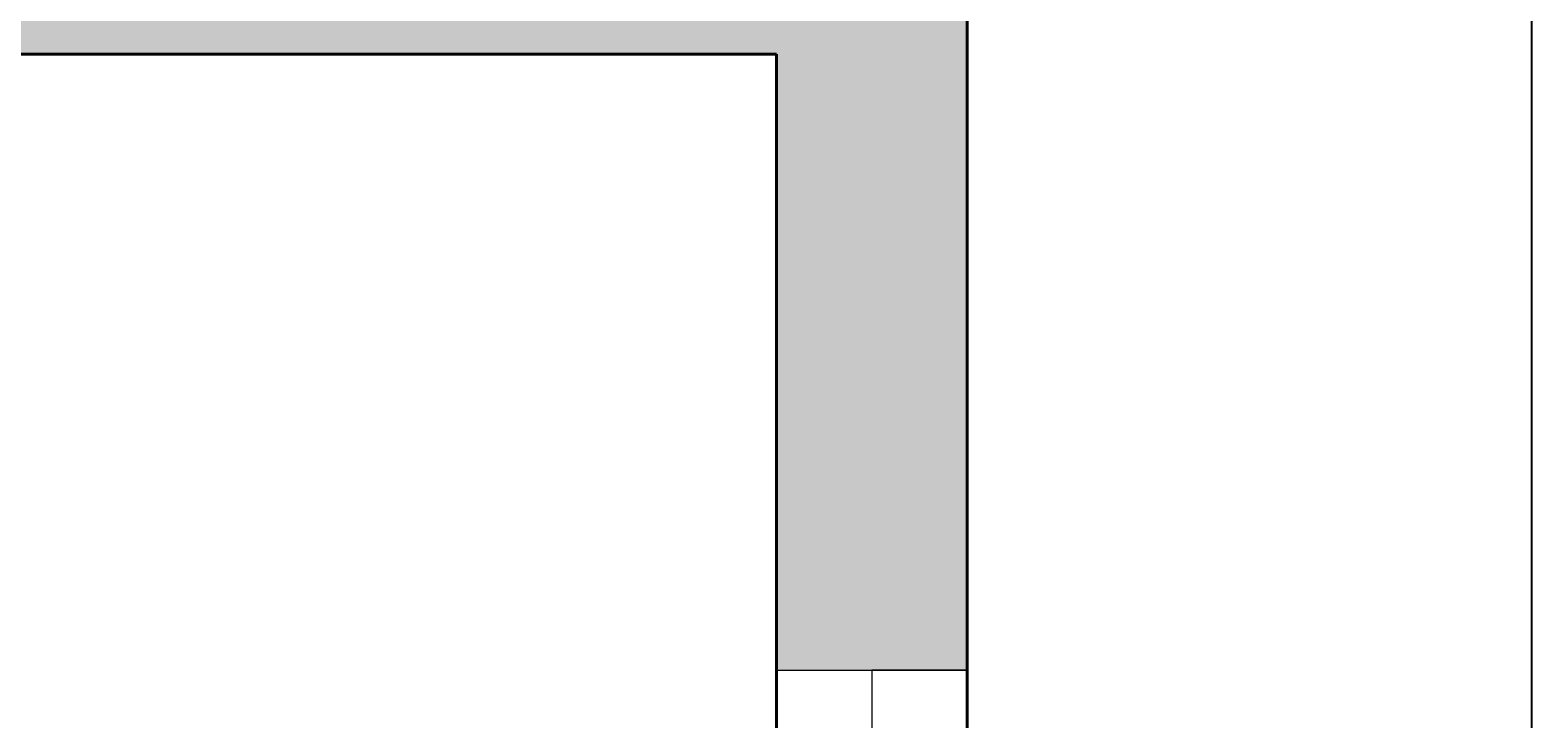
# Model space of a CAD drawing. Units: inches. Extents: x 1441 to 2460, y 1648 to 2683.
# Tile 20 of 35: x 1845 to 1916, y 2122 to 2154. Entities that reach past the tile are written whole.
import ezdxf

# ---------------------------------------------------------------- set-up
doc = ezdxf.new("R2010")
doc.units = ezdxf.units.IN
for name, color, linetype, lineweight in [('A-ANNO-DIMS', 2, 'Continuous', 18), ('A-GLAZ', 4, 'Continuous', 18), ('A-WALL', 7, 'Continuous', 40)]:
    doc.layers.add(name, color=color, linetype=linetype, lineweight=lineweight)
doc.layers.add('A-WALL-PATT', color=251, linetype='Continuous', lineweight=13, true_color=0x636466)
doc.styles.get("Standard").update_dxf_attribs({"font": 'arial.ttf'})
doc.dimstyles.get("Standard").update_dxf_attribs({"dimtxt": 0.18, "dimasz": 0.18, "dimexe": 0.18, "dimexo": 0.0625, "dimgap": 0.09, "dimtad": 0, "dimtih": 1, "dimtoh": 1, "dimdec": 4, "dimzin": 0, "dimdsep": 46, "dimtxsty": 'Standard', "dimcen": 0.09, "dimadec": 0, "dimazin": 0, "dimtfac": 1, "dimtdec": 4, "dimtofl": 0, "dimtmove": 0, "dimatfit": 3, "dimfxl": 1, "dimtolj": 1, "dimtzin": 0, "dimarcsym": 0})

# ---------------------------------------------------------------- blocks, each defined once
blk = doc.blocks.new('WIN-48-SASH')
for p, q in [((8.996, 48.001), (4.496, 48.001)), ((4.496, 48.001), (4.496, 0.001)), ((4.496, 0.001), (-0.004, 0.001))]:
    blk.add_line(p, q)
blk = doc.blocks.new('*D67')
at = {"layer": 'A-ANNO-DIMS', "color": 0, "lineweight": -2, "transparency": 16777216}
for p, q in [((1889.448, 2298.695), (1916.216, 2298.695)), ((1916.036, 2298.515), (1916.036, 2055.938)), ((1916.036, 1812.997), (1916.036, 2055.574)), ((1758.224, 1812.817), (1916.216, 1812.817))]:
    blk.add_line(p, q, dxfattribs=at)
at = {"layer": 'A-ANNO-DIMS', "color": 0, "transparency": 16777216}
for points in [[(1916.006, 2298.515), (1916.066, 2298.515), (1916.036, 2298.695)], [(1916.006, 1812.997), (1916.066, 1812.997), (1916.036, 1812.817)]]:
    blk.add_solid(points, dxfattribs=at)
at = {"layer": 'Defpoints', "color": 0, "transparency": 16777216}
for p in [(1889.386, 2298.695), (1916.036, 2298.695), (1758.161, 1812.817)]:
    blk.add_point(p, dxfattribs=at)
at = {"layer": 'A-ANNO-DIMS', "color": 0, "transparency": 16777216, "insert": (1916.036, 2055.756), "char_height": 0.18, "attachment_point": 5}
blk.add_mtext('\\A1;485.9', dxfattribs=at)

msp = doc.modelspace()

# ---------------------------------------------------------------- hatches: boundary and pattern name
at = {"layer": 'A-WALL-PATT'}
h = msp.add_hatch(color=256, dxfattribs=at)
h.dxf.hatch_style = 1
h.paths.add_polyline_path([(1627.5085, 2298.6952), (1568.8859, 2298.6952), (1568.8859, 2246.9605), (1577.8859, 2246.9605), (1577.8859, 2289.6952), (1627.5085, 2289.6952), (1627.5085, 2294.1952)])
h.paths.add_polyline_path([(1675.5777, 2298.6952), (1651.5085, 2298.6952), (1651.5085, 2289.6952), (1675.5777, 2289.6952), (1675.5777, 2294.1952)])
h.paths.add_polyline_path([(1667.3859, 2289.6952), (1662.8859, 2289.6952), (1662.8859, 2233.0622), (1667.3859, 2233.0622)])
h.paths.add_polyline_path([(1715.8721, 2294.3362), (1715.8721, 2295.2788), (1715.8721, 2298.6952), (1699.5777, 2298.6952), (1699.5777, 2289.6952), (1715.8721, 2289.6952)])
h.paths.add_polyline_path([(1707.8859, 2289.6952), (1703.3859, 2289.6952), (1703.3859, 2199.6952), (1707.8859, 2199.6952)])
h.paths.add_polyline_path([(1760.3859, 2204.637), (1755.8859, 2204.637), (1755.8859, 2199.6952), (1667.3859, 2199.6952), (1667.3859, 2204.637), (1662.8859, 2204.637), (1662.8859, 2195.1952), (1760.3859, 2195.1952)])
h.paths.add_polyline_path([(1760.3859, 2289.6952), (1755.8859, 2289.6952), (1755.8859, 2233.0622), (1760.3859, 2233.0622)])
h.paths.add_polyline_path([(1889.3859, 2298.6952), (1739.8721, 2298.6952), (1739.8721, 2289.6952), (1880.3859, 2289.6952), (1880.3859, 2250.8051), (1889.3859, 2250.8051)])
h.paths.add_polyline_path([(1889.3859, 2202.8051), (1880.3859, 2202.8051), (1880.3859, 2157.6952), (1747.948, 2157.6952), (1747.948, 2153.1952), (1755.8859, 2153.1952), (1755.8859, 2058.005), (1760.3859, 2058.005), (1760.3859, 2153.1952), (1880.3859, 2153.1952), (1880.3859, 2124.108), (1889.3859, 2124.108)])
h.paths.add_polyline_path([(1889.3859, 1984.8305), (1880.3859, 1984.8305), (1880.3859, 1834.1952), (1889.3859, 1834.1952)])
h.paths.add_polyline_path([(1889.3859, 2076.108), (1880.3859, 2076.108), (1880.3859, 2008.8305), (1889.3859, 2008.8305)])
h.paths.add_polyline_path([(1880.3859, 2027.1952), (1800.8859, 2027.1952), (1800.8859, 2000.9452), (1805.3859, 2000.9452), (1805.3859, 2022.6952), (1880.3859, 2022.6952)])
h.paths.add_polyline_path([(1800.8859, 2027.1952), (1760.3859, 2027.1952), (1760.3859, 2030.7912), (1755.8859, 2030.7912), (1755.8859, 2022.6952), (1800.8859, 2022.6952)])
h.paths.add_polyline_path([(1880.3859, 1974.6952), (1805.3859, 1974.6952), (1805.3859, 1978.7973), (1800.8859, 1978.7973), (1800.8859, 1974.6952), (1794.8823, 1974.6952), (1794.8823, 1970.1952), (1800.8859, 1970.1952), (1805.3859, 1970.1952), (1880.3859, 1970.1952)])
h.paths.add_polyline_path([(1760.3859, 1974.6952), (1755.8859, 1974.6952), (1755.8859, 1925.6952), (1751.8616, 1925.6952), (1751.8616, 1921.1952), (1760.3859, 1921.1952)])
h.paths.add_polyline_path([(1760.3859, 1921.1952), (1755.8859, 1921.1952), (1755.8859, 1843.1952), (1760.3859, 1843.1952)])
h.paths.add_polyline_path([(1799.1136, 1838.6952), (1799.1136, 1843.1952), (1760.3859, 1843.1952), (1751.8944, 1843.1952), (1751.8944, 1834.1952), (1758.1615, 1834.1952), (1799.1136, 1834.1952)])
h.paths.add_polyline_path([(1880.3859, 1843.1952), (1859.1136, 1843.1952), (1859.1136, 1834.1952), (1880.3859, 1834.1952)])
h.paths.add_polyline_path([(1577.8859, 1857.7914), (1568.8859, 1857.7914), (1568.8859, 1834.1952), (1695.0034, 1834.1952), (1695.0034, 1838.6952), (1695.0034, 1843.1952), (1577.8859, 1843.1952)])
h.paths.add_polyline_path([(1577.8859, 1959.2399), (1573.3859, 1959.2399), (1568.8859, 1959.2399), (1568.8859, 1905.7914), (1577.8859, 1905.7914), (1577.8859, 1921.1952), (1703.3859, 1921.1952), (1707.8859, 1921.1952), (1715.1501, 1921.1952), (1715.1501, 1925.6952), (1707.8859, 1925.6952), (1703.3859, 1925.6952), (1577.8859, 1925.6952)])
h.paths.add_polyline_path([(1577.8859, 2106.6907), (1568.8859, 2106.6907), (1568.8859, 2019.2399), (1577.8859, 2019.2399)])
h.paths.add_polyline_path([(1707.8859, 2051.6952), (1703.3859, 2051.6952), (1703.3859, 2048.6952), (1703.3859, 1925.6952), (1707.8859, 1925.6952)])
h.paths.add_polyline_path([(1703.3859, 2051.6952), (1676.3859, 2051.6952), (1676.3859, 2048.6952), (1703.3859, 2048.6952)])
h.paths.add_polyline_path([(1703.3859, 2102.6952), (1676.3859, 2102.6952), (1676.3859, 2099.6952), (1685.3859, 2099.6952), (1703.3859, 2099.6952)])
h.paths.add_polyline_path([(1707.8859, 2153.1952), (1710.5611, 2153.1952), (1710.5611, 2157.6952), (1707.8859, 2157.6952), (1707.8859, 2195.1952), (1703.3859, 2195.1952), (1703.3859, 2099.6952), (1707.8859, 2099.6952)])
h.paths.add_polyline_path([(1577.8859, 2198.9605), (1568.8859, 2198.9605), (1568.8859, 2166.6907), (1577.8859, 2166.6907)])

# ---------------------------------------------------------------- linework, layer by layer
at = {"layer": 'A-GLAZ'}
msp.add_line((1880.3859, 2124.108), (1889.3859, 2124.108), dxfattribs=at)
at = {"layer": 'A-WALL'}
for p, q in [((1889.3859, 2298.6952), (1889.3859, 1834.1952)), ((1760.3859, 2153.1952), (1880.3859, 2153.1952)), ((1880.3859, 2153.1952), (1880.3859, 1834.1952))]:
    msp.add_line(p, q, dxfattribs=at)

# ---------------------------------------------------------------- block references
at = {"layer": 'A-GLAZ'}
msp.add_blockref('WIN-48-SASH', (1880.39, 2076.1074), dxfattribs=at)

# ---------------------------------------------------------------- dimensions: what is measured, and where the dimension line sits
at = {"layer": 'A-ANNO-DIMS'}
dim = msp.add_linear_dim(base=(1916.0359, 2298.6952), p1=(1758.1615, 1812.8171), p2=(1889.3859, 2298.6952), angle=90, dimstyle='Standard', override={"dimdec": 1, "dimlfac": 1, "dimrnd": 0, "dimzin": 0, "dimdsep": 46, "dimlunit": 2}, dxfattribs=at)
dim.commit()
dim.dimension.update_dxf_attribs({"geometry": '*D67', "text_midpoint": (1916.0359, 2055.7561)})

doc.saveas('drawing.dxf')
